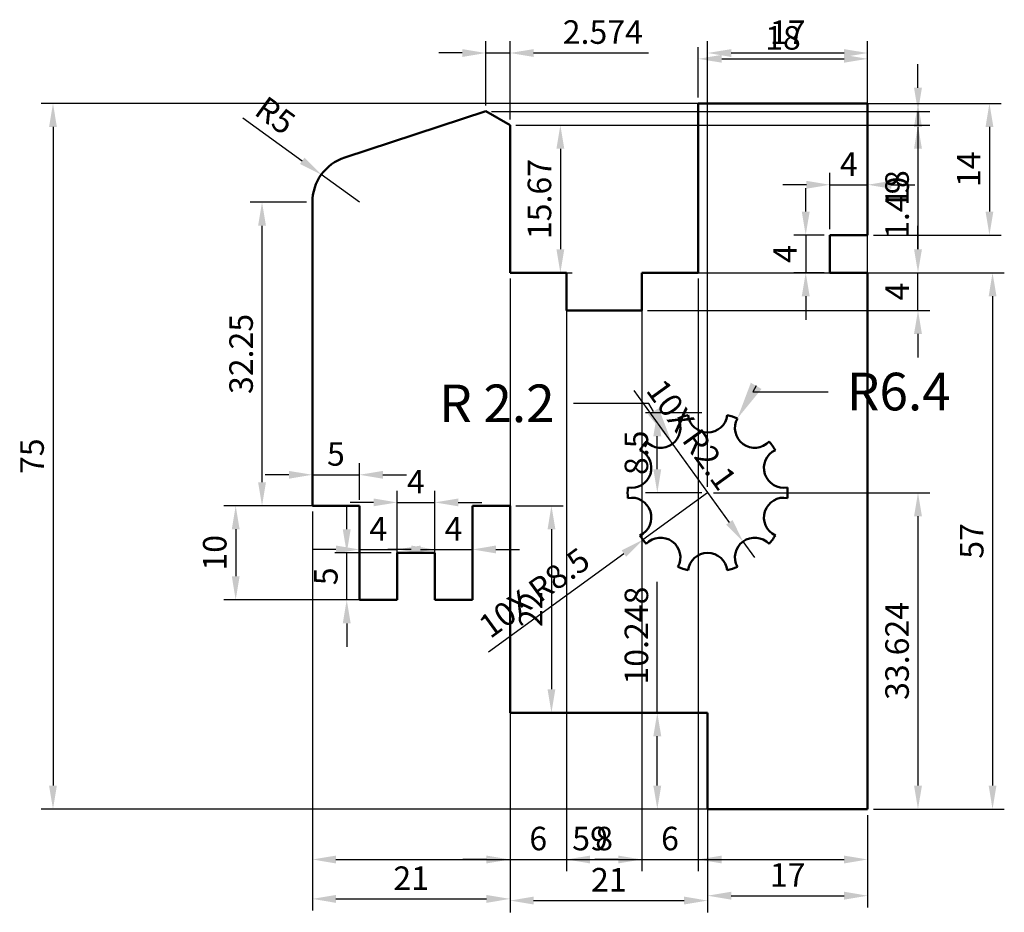
# Model space of a CAD drawing. Units: millimetres. Extents: x 3857 to 3961, y 1299 to 1394.
import ezdxf
from ezdxf import colors
from ezdxf.entities.mleader import LeaderData, LeaderLine
from ezdxf.math import Vec2, Vec3

# ---------------------------------------------------------------- set-up
doc = ezdxf.new("R2010")
doc.units = ezdxf.units.MM
doc.layers.add('M-DIMS', color=3, linetype='Continuous', lineweight=25)
doc.layers.add('M-OUTL', color=7, linetype='Continuous', lineweight=50)
doc.styles.get("Standard").update_dxf_attribs({"font": 'arial.ttf'})
doc.dimstyles.new('ISO-25', dxfattribs={"dimtxt": 2.5, "dimasz": 2.5, "dimexe": 1.25, "dimexo": 0.625, "dimtad": 1, "dimtxsty": 'Standard', "dimcen": 2.5, "dimadec": 0, "dimazin": 0, "dimtfac": 1, "dimtmove": 0, "dimatfit": 3, "dimfxl": 1, "dimarcsym": 0})

# ---------------------------------------------------------------- blocks, each defined once
blk = doc.blocks.new('*D1')
at = {"layer": 'Defpoints', "color": 0, "transparency": 16777216}
for p in [(3946.71, 1366.68), (3946.71, 1309.68), (3959.98, 1309.68)]:
    blk.add_point(p, dxfattribs=at)
at = {"layer": 'M-DIMS', "color": 0, "lineweight": -2, "transparency": 16777216}
for p, q in [((3947.33, 1366.68), (3961.23, 1366.68)), ((3959.98, 1364.18), (3959.98, 1312.18)), ((3947.33, 1309.68), (3961.23, 1309.68))]:
    blk.add_line(p, q, dxfattribs=at)
at = {"layer": 'M-DIMS', "color": 0, "transparency": 16777216}
for points in [[(3959.57, 1364.18), (3960.4, 1364.18), (3959.98, 1366.68)], [(3959.57, 1312.18), (3960.4, 1312.18), (3959.98, 1309.68)]]:
    blk.add_solid(points, dxfattribs=at)
at = {"layer": 'M-DIMS', "color": 0, "transparency": 16777216, "insert": (3958.09, 1338.18), "char_height": 2.5, "attachment_point": 5, "rotation": 90}
blk.add_mtext('57', dxfattribs=at)
blk = doc.blocks.new('*D2')
at = {"layer": 'Defpoints', "color": 0, "transparency": 16777216}
for p in [(3946.71, 1389.41), (3928.71, 1384.68), (3946.71, 1384.68)]:
    blk.add_point(p, dxfattribs=at)
at = {"layer": 'M-DIMS', "color": 0, "lineweight": -2, "transparency": 16777216}
for p, q in [((3928.71, 1385.3), (3928.71, 1390.66)), ((3946.71, 1385.3), (3946.71, 1390.66)), ((3931.21, 1389.41), (3944.21, 1389.41))]:
    blk.add_line(p, q, dxfattribs=at)
at = {"layer": 'M-DIMS', "color": 0, "transparency": 16777216}
for points in [[(3931.21, 1389.83), (3931.21, 1389), (3928.71, 1389.41)], [(3944.21, 1389.83), (3944.21, 1389), (3946.71, 1389.41)]]:
    blk.add_solid(points, dxfattribs=at)
at = {"layer": 'M-DIMS', "color": 0, "transparency": 16777216, "insert": (3937.71, 1391.31), "char_height": 2.5, "attachment_point": 5}
blk.add_mtext('18', dxfattribs=at)
blk = doc.blocks.new('*D3')
at = {"layer": 'Defpoints', "color": 0, "transparency": 16777216}
for p in [(3946.71, 1384.68), (3946.71, 1370.68), (3959.65, 1370.68)]:
    blk.add_point(p, dxfattribs=at)
at = {"layer": 'M-DIMS', "color": 0, "lineweight": -2, "transparency": 16777216}
for p, q in [((3947.33, 1384.68), (3960.9, 1384.68)), ((3959.65, 1382.18), (3959.65, 1373.18)), ((3947.33, 1370.68), (3960.9, 1370.68))]:
    blk.add_line(p, q, dxfattribs=at)
at = {"layer": 'M-DIMS', "color": 0, "transparency": 16777216}
for points in [[(3959.24, 1382.18), (3960.07, 1382.18), (3959.65, 1384.68)], [(3959.24, 1373.18), (3960.07, 1373.18), (3959.65, 1370.68)]]:
    blk.add_solid(points, dxfattribs=at)
at = {"layer": 'M-DIMS', "color": 0, "transparency": 16777216, "insert": (3957.77, 1377.68), "char_height": 2.5, "attachment_point": 5, "rotation": 90}
blk.add_mtext('14', dxfattribs=at)
blk = doc.blocks.new('*D4')
at = {"layer": 'Defpoints', "color": 0, "transparency": 16777216}
for p in [(3942.71, 1370.68), (3940.13, 1366.68), (3942.71, 1366.68)]:
    blk.add_point(p, dxfattribs=at)
at = {"layer": 'M-DIMS', "color": 0, "lineweight": -2, "transparency": 16777216}
for p, q in [((3940.13, 1373.18), (3940.13, 1375.68)), ((3942.08, 1370.68), (3938.88, 1370.68)), ((3940.13, 1370.68), (3940.13, 1366.68)), ((3942.08, 1366.68), (3938.88, 1366.68)), ((3940.13, 1364.18), (3940.13, 1361.68))]:
    blk.add_line(p, q, dxfattribs=at)
at = {"layer": 'M-DIMS', "color": 0, "transparency": 16777216}
for points in [[(3939.71, 1373.18), (3940.55, 1373.18), (3940.13, 1370.68)], [(3939.71, 1364.18), (3940.55, 1364.18), (3940.13, 1366.68)]]:
    blk.add_solid(points, dxfattribs=at)
at = {"layer": 'M-DIMS', "color": 0, "transparency": 16777216, "insert": (3938.26, 1368.68), "char_height": 2.5, "attachment_point": 5, "rotation": 90}
blk.add_mtext('4', dxfattribs=at)
blk = doc.blocks.new('*D5')
at = {"layer": 'Defpoints', "color": 0, "transparency": 16777216}
for p in [(3929.71, 1309.68), (3946.71, 1309.68), (3946.71, 1300.48)]:
    blk.add_point(p, dxfattribs=at)
at = {"layer": 'M-DIMS', "color": 0, "lineweight": -2, "transparency": 16777216}
for p, q in [((3929.71, 1309.05), (3929.71, 1299.23)), ((3946.71, 1309.05), (3946.71, 1299.23)), ((3932.21, 1300.48), (3944.21, 1300.48))]:
    blk.add_line(p, q, dxfattribs=at)
at = {"layer": 'M-DIMS', "color": 0, "transparency": 16777216}
for points in [[(3932.21, 1300.9), (3932.21, 1300.06), (3929.71, 1300.48)], [(3944.21, 1300.9), (3944.21, 1300.06), (3946.71, 1300.48)]]:
    blk.add_solid(points, dxfattribs=at)
at = {"layer": 'M-DIMS', "color": 0, "transparency": 16777216, "insert": (3938.21, 1302.36), "char_height": 2.5, "attachment_point": 5}
blk.add_mtext('17', dxfattribs=at)
blk = doc.blocks.new('*D6')
at = {"layer": 'Defpoints', "color": 0, "transparency": 16777216}
for p in [(3946.71, 1384.68), (3860.15, 1309.68), (3946.71, 1309.68)]:
    blk.add_point(p, dxfattribs=at)
at = {"layer": 'M-DIMS', "color": 0, "lineweight": -2, "transparency": 16777216}
for p, q in [((3946.08, 1384.68), (3858.9, 1384.68)), ((3860.15, 1382.18), (3860.15, 1312.18)), ((3946.08, 1309.68), (3858.9, 1309.68))]:
    blk.add_line(p, q, dxfattribs=at)
at = {"layer": 'M-DIMS', "color": 0, "transparency": 16777216}
for points in [[(3859.73, 1382.18), (3860.56, 1382.18), (3860.15, 1384.68)], [(3859.73, 1312.18), (3860.56, 1312.18), (3860.15, 1309.68)]]:
    blk.add_solid(points, dxfattribs=at)
at = {"layer": 'M-DIMS', "color": 0, "transparency": 16777216, "insert": (3858.25, 1347.18), "char_height": 2.5, "attachment_point": 5, "rotation": 90}
blk.add_mtext('75', dxfattribs=at)
blk = doc.blocks.new('*D7')
at = {"layer": 'Defpoints', "color": 0, "transparency": 16777216}
for p in [(3908.71, 1319.92), (3929.71, 1319.92), (3929.71, 1299.96)]:
    blk.add_point(p, dxfattribs=at)
at = {"layer": 'M-DIMS', "color": 0, "lineweight": -2, "transparency": 16777216}
for p, q in [((3908.71, 1319.3), (3908.71, 1298.71)), ((3929.71, 1319.3), (3929.71, 1298.71)), ((3911.21, 1299.96), (3927.21, 1299.96))]:
    blk.add_line(p, q, dxfattribs=at)
at = {"layer": 'M-DIMS', "color": 0, "transparency": 16777216}
for points in [[(3911.21, 1300.38), (3911.21, 1299.55), (3908.71, 1299.96)], [(3927.21, 1300.38), (3927.21, 1299.55), (3929.71, 1299.96)]]:
    blk.add_solid(points, dxfattribs=at)
at = {"layer": 'M-DIMS', "color": 0, "transparency": 16777216, "insert": (3919.21, 1301.85), "char_height": 2.5, "attachment_point": 5}
blk.add_mtext('21', dxfattribs=at)
blk = doc.blocks.new('*D8')
at = {"layer": 'Defpoints', "color": 0, "transparency": 16777216}
for p in [(3887.71, 1341.92), (3908.71, 1319.92), (3908.71, 1300.14)]:
    blk.add_point(p, dxfattribs=at)
at = {"layer": 'M-DIMS', "color": 0, "lineweight": -2, "transparency": 16777216}
for p, q in [((3887.71, 1341.3), (3887.71, 1298.89)), ((3908.71, 1319.3), (3908.71, 1298.89)), ((3890.21, 1300.14), (3906.21, 1300.14))]:
    blk.add_line(p, q, dxfattribs=at)
at = {"layer": 'M-DIMS', "color": 0, "transparency": 16777216}
for points in [[(3890.21, 1300.56), (3890.21, 1299.72), (3887.71, 1300.14)], [(3906.21, 1300.56), (3906.21, 1299.72), (3908.71, 1300.14)]]:
    blk.add_solid(points, dxfattribs=at)
at = {"layer": 'M-DIMS', "color": 0, "transparency": 16777216, "insert": (3898.21, 1302.02), "char_height": 2.5, "attachment_point": 5}
blk.add_mtext('21', dxfattribs=at)
blk = doc.blocks.new('*D9')
at = {"layer": 'Defpoints', "color": 0, "transparency": 16777216}
for p in [(3892.71, 1341.92), (3879.56, 1331.92), (3892.71, 1331.92)]:
    blk.add_point(p, dxfattribs=at)
at = {"layer": 'M-DIMS', "color": 0, "lineweight": -2, "transparency": 16777216}
for p, q in [((3892.08, 1341.92), (3878.31, 1341.92)), ((3879.56, 1339.42), (3879.56, 1334.42)), ((3892.08, 1331.92), (3878.31, 1331.92))]:
    blk.add_line(p, q, dxfattribs=at)
at = {"layer": 'M-DIMS', "color": 0, "transparency": 16777216}
for points in [[(3879.15, 1339.42), (3879.98, 1339.42), (3879.56, 1341.92)], [(3879.15, 1334.42), (3879.98, 1334.42), (3879.56, 1331.92)]]:
    blk.add_solid(points, dxfattribs=at)
at = {"layer": 'M-DIMS', "color": 0, "transparency": 16777216, "insert": (3877.66, 1336.92), "char_height": 2.5, "attachment_point": 5, "rotation": 90}
blk.add_mtext('10', dxfattribs=at)
blk = doc.blocks.new('*D10')
at = {"layer": 'Defpoints', "color": 0, "transparency": 16777216}
for p in [(3892.71, 1345.21), (3887.71, 1341.92), (3892.71, 1341.92)]:
    blk.add_point(p, dxfattribs=at)
at = {"layer": 'M-DIMS', "color": 0, "lineweight": -2, "transparency": 16777216}
for p, q in [((3887.71, 1342.55), (3887.71, 1346.46)), ((3892.71, 1342.55), (3892.71, 1346.46)), ((3885.21, 1345.21), (3882.71, 1345.21)), ((3887.71, 1345.21), (3892.71, 1345.21)), ((3895.21, 1345.21), (3897.71, 1345.21))]:
    blk.add_line(p, q, dxfattribs=at)
at = {"layer": 'M-DIMS', "color": 0, "transparency": 16777216}
for points in [[(3885.21, 1345.62), (3885.21, 1344.79), (3887.71, 1345.21)], [(3895.21, 1345.62), (3895.21, 1344.79), (3892.71, 1345.21)]]:
    blk.add_solid(points, dxfattribs=at)
at = {"layer": 'M-DIMS', "color": 0, "transparency": 16777216, "insert": (3890.21, 1347.1), "char_height": 2.5, "attachment_point": 5}
blk.add_mtext('5', dxfattribs=at)
blk = doc.blocks.new('*D11')
at = {"layer": 'Defpoints', "color": 0, "transparency": 16777216}
for p in [(3908.71, 1341.92), (3908.71, 1319.92), (3913.11, 1319.92)]:
    blk.add_point(p, dxfattribs=at)
at = {"layer": 'M-DIMS', "color": 0, "lineweight": -2, "transparency": 16777216}
for p, q in [((3909.33, 1341.92), (3914.36, 1341.92)), ((3913.11, 1339.42), (3913.11, 1322.42)), ((3909.33, 1319.92), (3914.36, 1319.92))]:
    blk.add_line(p, q, dxfattribs=at)
at = {"layer": 'M-DIMS', "color": 0, "transparency": 16777216}
for points in [[(3912.7, 1339.42), (3913.53, 1339.42), (3913.11, 1341.92)], [(3912.7, 1322.42), (3913.53, 1322.42), (3913.11, 1319.92)]]:
    blk.add_solid(points, dxfattribs=at)
at = {"layer": 'M-DIMS', "color": 0, "transparency": 16777216, "insert": (3911.23, 1330.92), "char_height": 2.5, "attachment_point": 5, "rotation": 90}
blk.add_mtext('22', dxfattribs=at)
blk = doc.blocks.new('*D12')
at = {"layer": 'Defpoints', "color": 0, "transparency": 16777216}
for p in [(3887.71, 1341.92), (3946.71, 1309.68), (3946.71, 1304.33)]:
    blk.add_point(p, dxfattribs=at)
at = {"layer": 'M-DIMS', "color": 0, "lineweight": -2, "transparency": 16777216}
for p, q in [((3887.71, 1341.3), (3887.71, 1303.08)), ((3946.71, 1309.05), (3946.71, 1303.08)), ((3890.21, 1304.33), (3944.21, 1304.33))]:
    blk.add_line(p, q, dxfattribs=at)
at = {"layer": 'M-DIMS', "color": 0, "transparency": 16777216}
for points in [[(3890.21, 1304.74), (3890.21, 1303.91), (3887.71, 1304.33)], [(3944.21, 1304.74), (3944.21, 1303.91), (3946.71, 1304.33)]]:
    blk.add_solid(points, dxfattribs=at)
at = {"layer": 'M-DIMS', "color": 0, "transparency": 16777216, "insert": (3917.21, 1306.23), "char_height": 2.5, "attachment_point": 5}
blk.add_mtext('59', dxfattribs=at)
blk = doc.blocks.new('*D13')
at = {"layer": 'Defpoints', "color": 0, "transparency": 16777216}
for p in [(3929.71, 1343.3), (3946.71, 1309.68), (3952.06, 1309.68)]:
    blk.add_point(p, dxfattribs=at)
at = {"layer": 'M-DIMS', "color": 0, "lineweight": -2, "transparency": 16777216}
for p, q in [((3930.33, 1343.3), (3953.31, 1343.3)), ((3952.06, 1340.8), (3952.06, 1312.18)), ((3947.33, 1309.68), (3953.31, 1309.68))]:
    blk.add_line(p, q, dxfattribs=at)
at = {"layer": 'M-DIMS', "color": 0, "transparency": 16777216}
for points in [[(3951.64, 1340.8), (3952.48, 1340.8), (3952.06, 1343.3)], [(3951.64, 1312.18), (3952.48, 1312.18), (3952.06, 1309.68)]]:
    blk.add_solid(points, dxfattribs=at)
at = {"layer": 'M-DIMS', "color": 0, "transparency": 16777216, "insert": (3950.16, 1326.49), "char_height": 2.5, "attachment_point": 5, "rotation": 90}
blk.add_mtext('33.624', dxfattribs=at)
blk = doc.blocks.new('*D14')
at = {"layer": 'Defpoints', "color": 0, "transparency": 16777216}
for p in [(3946.71, 1390.03), (3929.71, 1343.3), (3946.71, 1309.68)]:
    blk.add_point(p, dxfattribs=at)
at = {"layer": 'M-DIMS', "color": 0, "lineweight": -2, "transparency": 16777216}
for p, q in [((3929.71, 1343.93), (3929.71, 1391.28)), ((3946.71, 1310.3), (3946.71, 1391.28)), ((3932.21, 1390.03), (3944.21, 1390.03))]:
    blk.add_line(p, q, dxfattribs=at)
at = {"layer": 'M-DIMS', "color": 0, "transparency": 16777216}
for points in [[(3932.21, 1390.44), (3932.21, 1389.61), (3929.71, 1390.03)], [(3944.21, 1390.44), (3944.21, 1389.61), (3946.71, 1390.03)]]:
    blk.add_solid(points, dxfattribs=at)
at = {"layer": 'M-DIMS', "color": 0, "transparency": 16777216, "insert": (3938.21, 1391.91), "char_height": 2.5, "attachment_point": 5}
blk.add_mtext('17', dxfattribs=at)
blk = doc.blocks.new('*D15')
at = {"layer": 'Defpoints', "color": 0, "transparency": 16777216}
for p in [(3924.36, 1319.92), (3929.71, 1319.92), (3929.71, 1309.68)]:
    blk.add_point(p, dxfattribs=at)
at = {"layer": 'M-DIMS', "color": 0, "lineweight": -2, "transparency": 16777216}
for p, q in [((3924.36, 1319.92), (3924.36, 1333.82)), ((3929.08, 1319.92), (3923.11, 1319.92)), ((3924.36, 1312.18), (3924.36, 1317.42)), ((3929.08, 1309.68), (3923.11, 1309.68))]:
    blk.add_line(p, q, dxfattribs=at)
at = {"layer": 'M-DIMS', "color": 0, "transparency": 16777216}
for points in [[(3923.94, 1317.42), (3924.78, 1317.42), (3924.36, 1319.92)], [(3923.94, 1312.18), (3924.78, 1312.18), (3924.36, 1309.68)]]:
    blk.add_solid(points, dxfattribs=at)
at = {"layer": 'M-DIMS', "color": 0, "transparency": 16777216, "insert": (3922.46, 1328.12), "char_height": 2.5, "attachment_point": 5, "rotation": 90}
blk.add_mtext('10.248', dxfattribs=at)
blk = doc.blocks.new('*D16')
at = {"layer": 'Defpoints', "color": 0, "transparency": 16777216}
for p in [(3896.71, 1337.27), (3892.71, 1331.92), (3896.71, 1331.92)]:
    blk.add_point(p, dxfattribs=at)
at = {"layer": 'M-DIMS', "color": 0, "lineweight": -2, "transparency": 16777216}
for p, q in [((3892.71, 1332.55), (3892.71, 1338.52)), ((3896.71, 1332.55), (3896.71, 1338.52)), ((3890.21, 1337.27), (3887.71, 1337.27)), ((3892.71, 1337.27), (3896.71, 1337.27)), ((3899.21, 1337.27), (3901.71, 1337.27))]:
    blk.add_line(p, q, dxfattribs=at)
at = {"layer": 'M-DIMS', "color": 0, "transparency": 16777216}
for points in [[(3890.21, 1337.69), (3890.21, 1336.86), (3892.71, 1337.27)], [(3899.21, 1337.69), (3899.21, 1336.86), (3896.71, 1337.27)]]:
    blk.add_solid(points, dxfattribs=at)
at = {"layer": 'M-DIMS', "color": 0, "transparency": 16777216, "insert": (3894.71, 1339.15), "char_height": 2.5, "attachment_point": 5}
blk.add_mtext('4', dxfattribs=at)
blk = doc.blocks.new('*D17')
at = {"layer": 'Defpoints', "color": 0, "transparency": 16777216}
for p in [(3900.71, 1342.27), (3896.71, 1336.92), (3900.71, 1336.92)]:
    blk.add_point(p, dxfattribs=at)
at = {"layer": 'M-DIMS', "color": 0, "lineweight": -2, "transparency": 16777216}
for p, q in [((3896.71, 1337.55), (3896.71, 1343.52)), ((3900.71, 1337.55), (3900.71, 1343.52)), ((3894.21, 1342.27), (3891.71, 1342.27)), ((3896.71, 1342.27), (3900.71, 1342.27)), ((3903.21, 1342.27), (3905.71, 1342.27))]:
    blk.add_line(p, q, dxfattribs=at)
at = {"layer": 'M-DIMS', "color": 0, "transparency": 16777216}
for points in [[(3894.21, 1342.69), (3894.21, 1341.86), (3896.71, 1342.27)], [(3903.21, 1342.69), (3903.21, 1341.86), (3900.71, 1342.27)]]:
    blk.add_solid(points, dxfattribs=at)
at = {"layer": 'M-DIMS', "color": 0, "transparency": 16777216, "insert": (3898.71, 1344.15), "char_height": 2.5, "attachment_point": 5}
blk.add_mtext('4', dxfattribs=at)
blk = doc.blocks.new('*D18')
at = {"layer": 'Defpoints', "color": 0, "transparency": 16777216}
for p in [(3904.71, 1337.27), (3900.71, 1331.92), (3904.71, 1331.92)]:
    blk.add_point(p, dxfattribs=at)
at = {"layer": 'M-DIMS', "color": 0, "lineweight": -2, "transparency": 16777216}
for p, q in [((3900.71, 1332.55), (3900.71, 1338.52)), ((3904.71, 1332.55), (3904.71, 1338.52)), ((3898.21, 1337.27), (3895.71, 1337.27)), ((3900.71, 1337.27), (3904.71, 1337.27)), ((3907.21, 1337.27), (3909.71, 1337.27))]:
    blk.add_line(p, q, dxfattribs=at)
at = {"layer": 'M-DIMS', "color": 0, "transparency": 16777216}
for points in [[(3898.21, 1337.69), (3898.21, 1336.86), (3900.71, 1337.27)], [(3907.21, 1337.69), (3907.21, 1336.86), (3904.71, 1337.27)]]:
    blk.add_solid(points, dxfattribs=at)
at = {"layer": 'M-DIMS', "color": 0, "transparency": 16777216, "insert": (3902.71, 1339.15), "char_height": 2.5, "attachment_point": 5}
blk.add_mtext('4', dxfattribs=at)
blk = doc.blocks.new('*D19')
at = {"layer": 'Defpoints', "color": 0, "transparency": 16777216}
for p in [(3891.36, 1336.92), (3896.71, 1336.92), (3896.71, 1331.92)]:
    blk.add_point(p, dxfattribs=at)
at = {"layer": 'M-DIMS', "color": 0, "lineweight": -2, "transparency": 16777216}
for p, q in [((3891.36, 1339.42), (3891.36, 1341.92)), ((3896.08, 1336.92), (3890.11, 1336.92)), ((3891.36, 1331.92), (3891.36, 1336.92)), ((3896.08, 1331.92), (3890.11, 1331.92)), ((3891.36, 1329.42), (3891.36, 1326.92))]:
    blk.add_line(p, q, dxfattribs=at)
at = {"layer": 'M-DIMS', "color": 0, "transparency": 16777216}
for points in [[(3890.94, 1339.42), (3891.78, 1339.42), (3891.36, 1336.92)], [(3890.94, 1329.42), (3891.78, 1329.42), (3891.36, 1331.92)]]:
    blk.add_solid(points, dxfattribs=at)
at = {"layer": 'M-DIMS', "color": 0, "transparency": 16777216, "insert": (3889.46, 1334.42), "char_height": 2.5, "attachment_point": 5, "rotation": 90}
blk.add_mtext('5', dxfattribs=at)
blk = doc.blocks.new('*D20')
at = {"layer": 'Defpoints', "color": 0, "transparency": 16777216}
for p in [(3908.71, 1366.68), (3914.71, 1366.68), (3914.71, 1304.33)]:
    blk.add_point(p, dxfattribs=at)
at = {"layer": 'M-DIMS', "color": 0, "lineweight": -2, "transparency": 16777216}
for p, q in [((3908.71, 1366.05), (3908.71, 1303.08)), ((3914.71, 1366.05), (3914.71, 1303.08)), ((3906.21, 1304.33), (3903.71, 1304.33)), ((3908.71, 1304.33), (3914.71, 1304.33)), ((3917.21, 1304.33), (3919.71, 1304.33))]:
    blk.add_line(p, q, dxfattribs=at)
at = {"layer": 'M-DIMS', "color": 0, "transparency": 16777216}
for points in [[(3906.21, 1304.74), (3906.21, 1303.91), (3908.71, 1304.33)], [(3917.21, 1304.74), (3917.21, 1303.91), (3914.71, 1304.33)]]:
    blk.add_solid(points, dxfattribs=at)
at = {"layer": 'M-DIMS', "color": 0, "transparency": 16777216, "insert": (3911.71, 1306.23), "char_height": 2.5, "attachment_point": 5}
blk.add_mtext('6', dxfattribs=at)
blk = doc.blocks.new('*D21')
at = {"layer": 'Defpoints', "color": 0, "transparency": 16777216}
for p in [(3914.71, 1362.68), (3922.71, 1362.68), (3922.71, 1304.33)]:
    blk.add_point(p, dxfattribs=at)
at = {"layer": 'M-DIMS', "color": 0, "lineweight": -2, "transparency": 16777216}
for p, q in [((3914.71, 1362.05), (3914.71, 1303.08)), ((3922.71, 1362.05), (3922.71, 1303.08)), ((3917.21, 1304.33), (3920.21, 1304.33))]:
    blk.add_line(p, q, dxfattribs=at)
at = {"layer": 'M-DIMS', "color": 0, "transparency": 16777216}
for points in [[(3917.21, 1304.74), (3917.21, 1303.91), (3914.71, 1304.33)], [(3920.21, 1304.74), (3920.21, 1303.91), (3922.71, 1304.33)]]:
    blk.add_solid(points, dxfattribs=at)
at = {"layer": 'M-DIMS', "color": 0, "transparency": 16777216, "insert": (3918.71, 1306.23), "char_height": 2.5, "attachment_point": 5}
blk.add_mtext('8', dxfattribs=at)
blk = doc.blocks.new('*D22')
at = {"layer": 'Defpoints', "color": 0, "transparency": 16777216}
for p in [(3922.71, 1366.68), (3952.06, 1366.68), (3922.71, 1362.68)]:
    blk.add_point(p, dxfattribs=at)
at = {"layer": 'M-DIMS', "color": 0, "lineweight": -2, "transparency": 16777216}
for p, q in [((3952.06, 1369.18), (3952.06, 1371.68)), ((3923.33, 1366.68), (3953.31, 1366.68)), ((3952.06, 1362.68), (3952.06, 1366.68)), ((3923.33, 1362.68), (3953.31, 1362.68)), ((3952.06, 1360.18), (3952.06, 1357.68))]:
    blk.add_line(p, q, dxfattribs=at)
at = {"layer": 'M-DIMS', "color": 0, "transparency": 16777216}
for points in [[(3951.64, 1369.18), (3952.48, 1369.18), (3952.06, 1366.68)], [(3951.64, 1360.18), (3952.48, 1360.18), (3952.06, 1362.68)]]:
    blk.add_solid(points, dxfattribs=at)
at = {"layer": 'M-DIMS', "color": 0, "transparency": 16777216, "insert": (3950.18, 1364.68), "char_height": 2.5, "attachment_point": 5, "rotation": 90}
blk.add_mtext('4', dxfattribs=at)
blk = doc.blocks.new('*D23')
at = {"layer": 'Defpoints', "color": 0, "transparency": 16777216}
for p in [(3928.71, 1384.68), (3928.71, 1366.68), (3952.06, 1366.68)]:
    blk.add_point(p, dxfattribs=at)
at = {"layer": 'M-DIMS', "color": 0, "lineweight": -2, "transparency": 16777216}
for p, q in [((3929.33, 1384.68), (3953.31, 1384.68)), ((3952.06, 1382.18), (3952.06, 1369.18)), ((3929.33, 1366.68), (3953.31, 1366.68))]:
    blk.add_line(p, q, dxfattribs=at)
at = {"layer": 'M-DIMS', "color": 0, "transparency": 16777216}
for points in [[(3951.64, 1382.18), (3952.48, 1382.18), (3952.06, 1384.68)], [(3951.64, 1369.18), (3952.48, 1369.18), (3952.06, 1366.68)]]:
    blk.add_solid(points, dxfattribs=at)
at = {"layer": 'M-DIMS', "color": 0, "transparency": 16777216, "insert": (3950.16, 1375.68), "char_height": 2.5, "attachment_point": 5, "rotation": 90}
blk.add_mtext('18', dxfattribs=at)
blk = doc.blocks.new('*D24')
at = {"layer": 'Defpoints', "color": 0, "transparency": 16777216}
for p in [(3946.71, 1376.03), (3942.71, 1370.68), (3946.71, 1370.68)]:
    blk.add_point(p, dxfattribs=at)
at = {"layer": 'M-DIMS', "color": 0, "lineweight": -2, "transparency": 16777216}
for p, q in [((3942.71, 1371.3), (3942.71, 1377.28)), ((3946.71, 1371.3), (3946.71, 1377.28)), ((3940.21, 1376.03), (3937.71, 1376.03)), ((3942.71, 1376.03), (3946.71, 1376.03)), ((3949.21, 1376.03), (3951.71, 1376.03))]:
    blk.add_line(p, q, dxfattribs=at)
at = {"layer": 'M-DIMS', "color": 0, "transparency": 16777216}
for points in [[(3940.21, 1376.44), (3940.21, 1375.61), (3942.71, 1376.03)], [(3949.21, 1376.44), (3949.21, 1375.61), (3946.71, 1376.03)]]:
    blk.add_solid(points, dxfattribs=at)
at = {"layer": 'M-DIMS', "color": 0, "transparency": 16777216, "insert": (3944.71, 1377.9), "char_height": 2.5, "attachment_point": 5}
blk.add_mtext('4', dxfattribs=at)
blk = doc.blocks.new('*D25')
at = {"layer": 'Defpoints', "color": 0, "transparency": 16777216}
for p in [(3882.36, 1374.17), (3887.71, 1374.17), (3887.71, 1341.92)]:
    blk.add_point(p, dxfattribs=at)
at = {"layer": 'M-DIMS', "color": 0, "lineweight": -2, "transparency": 16777216}
for p, q in [((3887.08, 1374.17), (3881.11, 1374.17)), ((3882.36, 1344.42), (3882.36, 1371.67)), ((3887.08, 1341.92), (3881.11, 1341.92))]:
    blk.add_line(p, q, dxfattribs=at)
at = {"layer": 'M-DIMS', "color": 0, "transparency": 16777216}
for points in [[(3881.94, 1371.67), (3882.78, 1371.67), (3882.36, 1374.17)], [(3881.94, 1344.42), (3882.78, 1344.42), (3882.36, 1341.92)]]:
    blk.add_solid(points, dxfattribs=at)
at = {"layer": 'M-DIMS', "color": 0, "transparency": 16777216, "insert": (3880.46, 1358.05), "char_height": 2.5, "attachment_point": 5, "rotation": 90}
blk.add_mtext('32.25', dxfattribs=at)
blk = doc.blocks.new('*D26')
at = {"layer": 'Defpoints', "color": 0, "transparency": 16777216}
for p in [(3908.71, 1390.03), (3906.14, 1383.83), (3908.71, 1382.35)]:
    blk.add_point(p, dxfattribs=at)
at = {"layer": 'M-DIMS', "color": 0, "lineweight": -2, "transparency": 16777216}
for p, q in [((3906.14, 1384.46), (3906.14, 1391.28)), ((3908.71, 1382.97), (3908.71, 1391.28)), ((3903.64, 1390.03), (3901.14, 1390.03)), ((3906.14, 1390.03), (3908.71, 1390.03)), ((3911.21, 1390.03), (3923.43, 1390.03))]:
    blk.add_line(p, q, dxfattribs=at)
at = {"layer": 'M-DIMS', "color": 0, "transparency": 16777216}
for points in [[(3903.64, 1390.44), (3903.64, 1389.61), (3906.14, 1390.03)], [(3911.21, 1390.44), (3911.21, 1389.61), (3908.71, 1390.03)]]:
    blk.add_solid(points, dxfattribs=at)
at = {"layer": 'M-DIMS', "color": 0, "transparency": 16777216, "insert": (3918.57, 1391.93), "char_height": 2.5, "attachment_point": 5}
blk.add_mtext('2.574', dxfattribs=at)
blk = doc.blocks.new('*D27')
at = {"layer": 'Defpoints', "color": 0, "transparency": 16777216}
for p in [(3906.14, 1383.83), (3908.71, 1382.35), (3952.06, 1382.35)]:
    blk.add_point(p, dxfattribs=at)
at = {"layer": 'M-DIMS', "color": 0, "lineweight": -2, "transparency": 16777216}
for p, q in [((3952.06, 1386.33), (3952.06, 1388.83)), ((3906.76, 1383.83), (3953.31, 1383.83)), ((3952.06, 1383.83), (3952.06, 1382.35)), ((3909.33, 1382.35), (3953.31, 1382.35)), ((3952.06, 1379.85), (3952.06, 1369.83))]:
    blk.add_line(p, q, dxfattribs=at)
at = {"layer": 'M-DIMS', "color": 0, "transparency": 16777216}
for points in [[(3951.64, 1386.33), (3952.48, 1386.33), (3952.06, 1383.83)], [(3951.64, 1379.85), (3952.48, 1379.85), (3952.06, 1382.35)]]:
    blk.add_solid(points, dxfattribs=at)
at = {"layer": 'M-DIMS', "color": 0, "transparency": 16777216, "insert": (3950.16, 1373.59), "char_height": 2.5, "attachment_point": 5, "rotation": 90}
blk.add_mtext('1.49', dxfattribs=at)
blk = doc.blocks.new('*D28')
at = {"layer": 'Defpoints', "color": 0, "transparency": 16777216}
for p in [(3908.71, 1382.35), (3908.71, 1366.68), (3914.06, 1366.68)]:
    blk.add_point(p, dxfattribs=at)
at = {"layer": 'M-DIMS', "color": 0, "lineweight": -2, "transparency": 16777216}
for p, q in [((3909.33, 1382.35), (3915.31, 1382.35)), ((3914.06, 1379.85), (3914.06, 1369.18)), ((3909.33, 1366.68), (3915.31, 1366.68))]:
    blk.add_line(p, q, dxfattribs=at)
at = {"layer": 'M-DIMS', "color": 0, "transparency": 16777216}
for points in [[(3913.64, 1379.85), (3914.48, 1379.85), (3914.06, 1382.35)], [(3913.64, 1369.18), (3914.48, 1369.18), (3914.06, 1366.68)]]:
    blk.add_solid(points, dxfattribs=at)
at = {"layer": 'M-DIMS', "color": 0, "transparency": 16777216, "insert": (3912.16, 1374.51), "char_height": 2.5, "attachment_point": 5, "rotation": 90}
blk.add_mtext('15.67', dxfattribs=at)
blk = doc.blocks.new('*D29')
at = {"layer": 'Defpoints', "color": 0, "transparency": 16777216}
for p in [(3922.71, 1366.68), (3928.71, 1366.68), (3928.71, 1304.33)]:
    blk.add_point(p, dxfattribs=at)
at = {"layer": 'M-DIMS', "color": 0, "lineweight": -2, "transparency": 16777216}
for p, q in [((3922.71, 1366.05), (3922.71, 1303.08)), ((3928.71, 1366.05), (3928.71, 1303.08)), ((3920.21, 1304.33), (3917.71, 1304.33)), ((3922.71, 1304.33), (3928.71, 1304.33)), ((3931.21, 1304.33), (3933.71, 1304.33))]:
    blk.add_line(p, q, dxfattribs=at)
at = {"layer": 'M-DIMS', "color": 0, "transparency": 16777216}
for points in [[(3920.21, 1304.74), (3920.21, 1303.91), (3922.71, 1304.33)], [(3931.21, 1304.74), (3931.21, 1303.91), (3928.71, 1304.33)]]:
    blk.add_solid(points, dxfattribs=at)
at = {"layer": 'M-DIMS', "color": 0, "transparency": 16777216, "insert": (3925.71, 1306.23), "char_height": 2.5, "attachment_point": 5}
blk.add_mtext('6', dxfattribs=at)
blk = doc.blocks.new('*D30')
at = {"layer": 'Defpoints', "color": 0, "transparency": 16777216}
for p in [(3924.36, 1351.8), (3929.71, 1351.8), (3929.71, 1343.3)]:
    blk.add_point(p, dxfattribs=at)
at = {"layer": 'M-DIMS', "color": 0, "lineweight": -2, "transparency": 16777216}
for p, q in [((3929.08, 1351.8), (3923.11, 1351.8)), ((3924.36, 1345.8), (3924.36, 1349.3)), ((3929.08, 1343.3), (3923.11, 1343.3))]:
    blk.add_line(p, q, dxfattribs=at)
at = {"layer": 'M-DIMS', "color": 0, "transparency": 16777216}
for points in [[(3923.94, 1349.3), (3924.78, 1349.3), (3924.36, 1351.8)], [(3923.94, 1345.8), (3924.78, 1345.8), (3924.36, 1343.3)]]:
    blk.add_solid(points, dxfattribs=at)
at = {"layer": 'M-DIMS', "color": 0, "transparency": 16777216, "insert": (3922.46, 1347.55), "char_height": 2.5, "attachment_point": 5, "rotation": 90}
blk.add_mtext('8.5', dxfattribs=at)
blk = doc.blocks.new('*D31')
at = {"layer": 'Defpoints', "color": 0, "transparency": 16777216}
for p in [(3888.66, 1377.11), (3892.71, 1374.17)]:
    blk.add_point(p, dxfattribs=at)
at = {"layer": 'M-DIMS', "color": 0, "lineweight": -2, "transparency": 16777216}
for p, q in [((3880.32, 1383.15), (3886.64, 1378.57)), ((3892.71, 1374.17), (3888.66, 1377.11))]:
    blk.add_line(p, q, dxfattribs=at)
at = {"layer": 'M-DIMS', "color": 0, "transparency": 16777216}
blk.add_solid([(3886.88, 1378.91), (3886.39, 1378.24), (3888.66, 1377.11)], dxfattribs=at)
at = {"layer": 'M-DIMS', "color": 0, "transparency": 16777216, "insert": (3883.58, 1383.13), "char_height": 2.5, "attachment_point": 5, "rotation": 324.0676}
blk.add_mtext('R5', dxfattribs=at)
blk = doc.blocks.new('*D32')
at = {"layer": 'Defpoints', "color": 0, "transparency": 16777216}
for p in [(3929.71, 1343.3), (3922.83, 1338.3)]:
    blk.add_point(p, dxfattribs=at)
at = {"layer": 'M-DIMS', "color": 0, "lineweight": -2, "transparency": 16777216}
for p, q in [((3929.71, 1343.3), (3922.83, 1338.3)), ((3906.42, 1326.38), (3920.81, 1336.84))]:
    blk.add_line(p, q, dxfattribs=at)
at = {"layer": 'M-DIMS', "color": 0, "transparency": 16777216}
blk.add_solid([(3920.57, 1337.17), (3921.06, 1336.5), (3922.83, 1338.3)], dxfattribs=at)
at = {"layer": 'M-DIMS', "color": 0, "transparency": 16777216, "insert": (3911.48, 1332.41), "char_height": 2.5, "attachment_point": 5, "rotation": 35.9989}
blk.add_mtext('10X R8.5', dxfattribs=at)
blk = doc.blocks.new('*D33')
at = {"layer": 'Defpoints', "color": 0, "transparency": 16777216}
for p in [(3933.47, 1338.13), (3934.71, 1336.42)]:
    blk.add_point(p, dxfattribs=at)
at = {"layer": 'M-DIMS', "color": 0, "lineweight": -2, "transparency": 16777216}
for p, q in [((3921.87, 1354.16), (3932.01, 1340.15)), ((3934.71, 1336.42), (3933.47, 1338.13))]:
    blk.add_line(p, q, dxfattribs=at)
at = {"layer": 'M-DIMS', "color": 0, "transparency": 16777216}
blk.add_solid([(3932.35, 1340.4), (3931.67, 1339.91), (3933.47, 1338.13)], dxfattribs=at)
at = {"layer": 'M-DIMS', "color": 0, "transparency": 16777216, "insert": (3927.75, 1349.28), "char_height": 2.5, "attachment_point": 5, "rotation": 305.897}
blk.add_mtext('10X R2.1', dxfattribs=at)

msp = doc.modelspace()

# ---------------------------------------------------------------- linework, layer by layer
at = {"layer": 'M-OUTL'}
for p, q in [((3946.7097, 1384.6771), (3928.7097, 1384.6771)), ((3928.7097, 1384.6771), (3928.7097, 1366.6771)), ((3946.7097, 1370.6771), (3946.7097, 1384.6771)), ((3906.1355, 1383.8336), (3891.1528, 1378.9241)), ((3908.7097, 1382.3474), (3906.1355, 1383.8336)), ((3908.7097, 1366.6771), (3908.7097, 1382.3474)), ((3887.7097, 1341.9249), (3887.7097, 1374.1727)), ((3942.7097, 1366.6771), (3942.7097, 1370.6771)), ((3942.7097, 1370.6771), (3946.7097, 1370.6771)), ((3914.7097, 1366.6771), (3908.7097, 1366.6771)), ((3914.7097, 1362.6771), (3914.7097, 1366.6771)), ((3928.7097, 1366.6771), (3922.7097, 1366.6771)), ((3922.7097, 1366.6771), (3922.7097, 1362.6771)), ((3946.7097, 1366.6771), (3942.7097, 1366.6771)), ((3946.7097, 1309.6771), (3946.7097, 1366.6771)), ((3922.7097, 1362.6771), (3914.7097, 1362.6771)), ((3887.7097, 1341.9249), (3892.7097, 1341.9249)), ((3892.7097, 1341.9249), (3892.7097, 1331.9249)), ((3904.7097, 1331.9249), (3904.7097, 1341.9249)), ((3904.7097, 1341.9249), (3908.7097, 1341.9249)), ((3908.7097, 1319.9249), (3908.7097, 1341.9249)), ((3908.7097, 1341.9249), (3908.7097, 1319.9249)), ((3896.7097, 1331.9249), (3896.7097, 1336.9249)), ((3896.7097, 1336.9249), (3900.7097, 1336.9249)), ((3900.7097, 1336.9249), (3900.7097, 1331.9249)), ((3892.7097, 1331.9249), (3896.7097, 1331.9249)), ((3900.7097, 1331.9249), (3904.7097, 1331.9249)), ((3908.7097, 1319.9249), (3929.7097, 1319.9249)), ((3929.7097, 1319.9249), (3929.7097, 1309.6771)), ((3946.7097, 1309.6771), (3929.7097, 1309.6771))]:
    msp.add_line(p, q, dxfattribs=at)
for centre, radius, start, end in [((3892.7097, 1374.1727), 5, 108.142766, 180), ((3924.7135, 1350.1777), 2.1, 223.095839, 28.904161), ((3929.7097, 1343.301), 8.5, 104.191678, 111.808322), ((3929.7097, 1351.801), 2.1, 187.095839, 352.904161), ((3929.7097, 1343.301), 8.5, 68.191678, 75.808322), ((3934.7059, 1350.1777), 2.1, 151.095839, 316.904161), ((3929.7097, 1343.301), 8.5, 140.191678, 147.808322), ((3929.7097, 1343.301), 8.5, 32.191678, 39.808322), ((3921.6257, 1345.9277), 2.1, 259.095839, 64.904161), ((3937.7937, 1345.9277), 2.1, 115.095839, 280.904161), ((3929.7097, 1343.301), 8.5, 176.191678, 183.808322), ((3929.7097, 1343.301), 8.5, 356.191678, 3.808322), ((3921.6257, 1340.6744), 2.1, 295.095839, 100.904161), ((3937.7937, 1340.6744), 2.1, 79.095839, 244.904161), ((3929.7097, 1343.301), 8.5, 212.191678, 219.808322), ((3924.7135, 1336.4244), 2.1, 331.095839, 136.904161), ((3934.7059, 1336.4244), 2.1, 43.095839, 208.904161), ((3929.7097, 1343.301), 8.5, 320.191678, 327.808322), ((3929.7097, 1334.801), 2.1, 7.095839, 172.904161), ((3929.7097, 1343.301), 8.5, 248.191678, 255.808322), ((3929.7097, 1343.301), 8.5, 284.191678, 291.808322)]:
    msp.add_arc(centre, radius, start, end, dxfattribs=at)

# ---------------------------------------------------------------- dimensions: what is measured, and where the dimension line sits
at = {"layer": 'M-DIMS'}
for base, p1, p2, override, picture, middle in [((3908.7097, 1390.0271), (3906.1355, 1383.8336), (3908.7097, 1382.3474), {"dimdec": 3, "dimlfac": 1, "dimrnd": 0, "dimzin": 0, "dimdsep": 46, "dimlunit": 2}, '*D26', (3918.569, 1391.9286)), ((3946.7097, 1389.4131), (3928.7097, 1384.6771), (3946.7097, 1384.6771), {"dimclrd": 0, "dimclre": 0, "dimclrt": 0}, '*D2', (3937.7097, 1391.3146)), ((3946.7097, 1390.0271), (3929.7097, 1343.301), (3946.7097, 1309.6771), {"dimdec": 0, "dimlfac": 1, "dimrnd": 0, "dimzin": 0, "dimdsep": 46, "dimlunit": 2}, '*D14', (3938.2097, 1391.9073)), ((3946.7097, 1376.0271), (3942.7097, 1370.6771), (3946.7097, 1370.6771), {"dimdec": 0, "dimlfac": 1, "dimrnd": 0, "dimzin": 0, "dimdsep": 46, "dimlunit": 2}, '*D24', (3944.7097, 1377.9021)), ((3914.7097, 1304.3271), (3908.7097, 1366.6771), (3914.7097, 1366.6771), {"dimdec": 0, "dimlfac": 1, "dimrnd": 0, "dimzin": 0, "dimdsep": 46, "dimlunit": 2}, '*D20', (3911.7097, 1306.2286)), ((3928.7097, 1304.3271), (3922.7097, 1366.6771), (3928.7097, 1366.6771), {"dimdec": 0, "dimlfac": 1, "dimrnd": 0, "dimzin": 0, "dimdsep": 46, "dimlunit": 2}, '*D29', (3925.7097, 1306.2286)), ((3922.7097, 1304.3271), (3914.7097, 1362.6771), (3922.7097, 1362.6771), {"dimdec": 0, "dimlfac": 1, "dimrnd": 0, "dimzin": 0, "dimdsep": 46, "dimlunit": 2}, '*D21', (3918.7097, 1306.2286)), ((3892.7097, 1345.2065), (3887.7097, 1341.9249), (3892.7097, 1341.9249), {"dimclrd": 0, "dimclre": 0, "dimclrt": 0}, '*D10', (3890.2097, 1347.1028)), ((3900.7097, 1342.2749), (3896.7097, 1336.9249), (3900.7097, 1336.9249), {"dimdec": 0, "dimlfac": 1, "dimrnd": 0, "dimzin": 0, "dimdsep": 46, "dimlunit": 2}, '*D17', (3898.7097, 1344.1499)), ((3908.7097, 1300.1399), (3887.7097, 1341.9249), (3908.7097, 1319.9249), {"dimclrd": 0, "dimclre": 0, "dimclrt": 0}, '*D8', (3898.2097, 1302.02)), ((3946.7097, 1304.3271), (3887.7097, 1341.9249), (3946.7097, 1309.6771), {"dimdec": 0, "dimlfac": 1, "dimrnd": 0, "dimzin": 0, "dimdsep": 46, "dimlunit": 2}, '*D12', (3917.2097, 1306.2286)), ((3896.7097, 1337.2749), (3892.7097, 1331.9249), (3896.7097, 1331.9249), {"dimdec": 0, "dimlfac": 1, "dimrnd": 0, "dimzin": 0, "dimdsep": 46, "dimlunit": 2}, '*D16', (3894.7097, 1339.1499)), ((3904.7097, 1337.2749), (3900.7097, 1331.9249), (3904.7097, 1331.9249), {"dimdec": 0, "dimlfac": 1, "dimrnd": 0, "dimzin": 0, "dimdsep": 46, "dimlunit": 2}, '*D18', (3902.7097, 1339.1499)), ((3929.7097, 1299.965), (3908.7097, 1319.9249), (3929.7097, 1319.9249), {"dimclrd": 0, "dimclre": 0, "dimclrt": 0}, '*D7', (3919.2097, 1301.8451)), ((3946.7097, 1300.4815), (3929.7097, 1309.6771), (3946.7097, 1309.6771), {"dimclrd": 0, "dimclre": 0, "dimclrt": 0}, '*D5', (3938.2097, 1302.3616))]:
    dim = msp.add_linear_dim(base=base, p1=p1, p2=p2, dimstyle='ISO-25', override=override, dxfattribs=at)
    dim.commit()
    dim.dimension.update_dxf_attribs({"geometry": picture, "text_midpoint": middle})
for base, p1, p2, angle, override, picture, middle in [((3952.0597, 1382.3474), (3906.1355, 1383.8336), (3908.7097, 1382.3474), 90, {"dimdec": 2, "dimlfac": 1, "dimrnd": 0, "dimzin": 0, "dimdsep": 46, "dimlunit": 2}, '*D27', (3950.1583, 1373.5906)), ((3860.1472, 1309.6771), (3946.7097, 1384.6771), (3946.7097, 1309.6771), 90, {"dimclrd": 0, "dimclre": 0, "dimclrt": 0}, '*D6', (3858.2509, 1347.1771)), ((3952.0597, 1366.6771), (3928.7097, 1384.6771), (3928.7097, 1366.6771), 90, {"dimdec": 0, "dimlfac": 1, "dimrnd": 0, "dimzin": 0, "dimdsep": 46, "dimlunit": 2}, '*D23', (3950.1583, 1375.6771)), ((3959.6549, 1370.6771), (3946.7097, 1384.6771), (3946.7097, 1370.6771), 90, {"dimclrd": 0, "dimclre": 0, "dimclrt": 0}, '*D3', (3957.7748, 1377.6771)), ((3914.0597, 1366.6771), (3908.7097, 1382.3474), (3908.7097, 1366.6771), 270, {"dimdec": 2, "dimlfac": 1, "dimrnd": 0, "dimzin": 0, "dimdsep": 46, "dimlunit": 2}, '*D28', (3912.1583, 1374.5123)), ((3940.1303, 1366.6771), (3942.7097, 1370.6771), (3942.7097, 1366.6771), 90, {"dimclrd": 0, "dimclre": 0, "dimclrt": 0}, '*D4', (3938.2553, 1368.6771)), ((3882.3597, 1374.1727), (3887.7097, 1341.9249), (3887.7097, 1374.1727), 90, {"dimdec": 2, "dimlfac": 1, "dimrnd": 0, "dimzin": 0, "dimdsep": 46, "dimlunit": 2}, '*D25', (3880.4574, 1358.0488)), ((3952.0597, 1366.6771), (3922.7097, 1362.6771), (3922.7097, 1366.6771), 90, {"dimdec": 0, "dimlfac": 1, "dimrnd": 0, "dimzin": 0, "dimdsep": 46, "dimlunit": 2}, '*D22', (3950.1847, 1364.6771)), ((3959.9818, 1309.6771), (3946.7097, 1366.6771), (3946.7097, 1309.6771), 90, {"dimclrd": 0, "dimclre": 0, "dimclrt": 0}, '*D1', (3958.0854, 1338.1771)), ((3924.3597, 1351.801), (3929.7097, 1343.301), (3929.7097, 1351.801), 90, {"dimdec": 1, "dimlfac": 1, "dimrnd": 0, "dimzin": 0, "dimdsep": 46, "dimlunit": 2}, '*D30', (3922.4583, 1347.551)), ((3952.0597, 1309.6771), (3929.7097, 1343.301), (3946.7097, 1309.6771), 90, {"dimdec": 3, "dimlfac": 1, "dimrnd": 0, "dimzin": 0, "dimdsep": 46, "dimlunit": 2}, '*D13', (3950.1574, 1326.4891)), ((3879.5623, 1331.9249), (3892.7097, 1341.9249), (3892.7097, 1331.9249), 90, {"dimclrd": 0, "dimclre": 0, "dimclrt": 0}, '*D9', (3877.6608, 1336.9249)), ((3891.3597, 1336.9249), (3896.7097, 1331.9249), (3896.7097, 1336.9249), 90, {"dimdec": 0, "dimlfac": 1, "dimrnd": 0, "dimzin": 0, "dimdsep": 46, "dimlunit": 2}, '*D19', (3889.4634, 1334.4249)), ((3913.1123, 1319.9249), (3908.7097, 1341.9249), (3908.7097, 1319.9249), 90, {"dimclrd": 0, "dimclre": 0, "dimclrt": 0}, '*D11', (3911.2321, 1330.9249)), ((3924.3597, 1319.9249), (3929.7097, 1309.6771), (3929.7097, 1319.9249), 90, {"dimdec": 3, "dimlfac": 1, "dimrnd": 0, "dimzin": 0, "dimdsep": 46, "dimlunit": 2}, '*D15', (3922.4583, 1328.1241))]:
    dim = msp.add_linear_dim(base=base, p1=p1, p2=p2, angle=angle, dimstyle='ISO-25', override=override, dxfattribs=at)
    dim.commit()
    dim.dimension.update_dxf_attribs({"geometry": picture, "text_midpoint": middle})
dim = msp.add_radius_dim(center=(3892.7097, 1374.1727), mpoint=(3888.6612, 1377.1069), dimstyle='ISO-25', override={"dimdec": 0, "dimlfac": 1, "dimrnd": 0, "dimzin": 0, "dimdsep": 46, "dimlunit": 2}, dxfattribs=at)
dim.commit()
dim.dimension.update_dxf_attribs({"geometry": '*D31', "text_midpoint": (3883.5796, 1383.1316)})
for center, mpoint, picture, middle in [((3934.7059, 1336.4244), (3933.4746, 1338.1255), '*D33', (3927.7473, 1349.2814)), ((3929.7097, 1343.301), (3922.833, 1338.305), '*D32', (3911.4846, 1332.4105))]:
    dim = msp.add_radius_dim(center=center, mpoint=mpoint, text='10X <>', dimstyle='ISO-25', override={"dimdec": 1, "dimlfac": 1, "dimrnd": 0, "dimzin": 0, "dimdsep": 46, "dimlunit": 2}, dxfattribs=at)
    dim.commit()
    dim.dimension.update_dxf_attribs({"geometry": picture, "text_midpoint": middle})

# ---------------------------------------------------------------- leaders
ml = msp.add_multileader_mtext('Standard', dxfattribs=at)
ml.set_content('R6.4', color=256)
ml.set_leader_properties()
ml.build(insert=Vec2(0, 0))
ctx = ml.context
ctx.base_point, ctx.plane_origin = Vec3(3942.4987, 1354.018), Vec3(3932.8675, 1351.1927)
notes = []
notes.append((ctx, [(0, (1, 1, 0), (3934.4987, 1354.018), (1, 0), 8, [(0, [(3932.8675, 1351.1927)], 0, [])])]))
ctx.mtext.insert, ctx.mtext.flow_direction = Vec3(3944.4987, 1356.0521), 5
ml = msp.add_multileader_mtext('Standard', dxfattribs=at)
ml.set_content('R 2.2', color=256)
ml.set_leader_properties()
ml.build(insert=Vec2(0, 0))
ctx = ml.context
ctx.base_point, ctx.plane_origin = Vec3(3898.8304, 1352.8008), Vec3(3925.9479, 1348.4787)
ctx.text_align_type = 2
notes.append((ctx, [(0, (1, 1, 0), (3923.4525, 1352.8008), (-1, 0), 8, [(0, [(3925.9479, 1348.4787)], 0, [])])]))
ctx.mtext.insert, ctx.mtext.alignment, ctx.mtext.flow_direction = Vec3(3913.4525, 1354.8022), 3, 5
for ctx, leaders in notes:
    for number, flags, end, landing, length, lines in leaders:
        leader = LeaderData()
        leader.index, (leader.has_last_leader_line, leader.has_dogleg_vector, leader.attachment_direction) = number, flags
        leader.last_leader_point, leader.dogleg_vector, leader.dogleg_length = Vec3(end), Vec3(landing), length
        for number, points, colour, breaks in lines:
            line = LeaderLine()
            line.index, line.vertices, line.color, line.breaks = number, Vec3.list(points), colors.encode_raw_color(colour), breaks
            leader.lines.append(line)
        ctx.leaders.append(leader)

doc.saveas('drawing.dxf')
